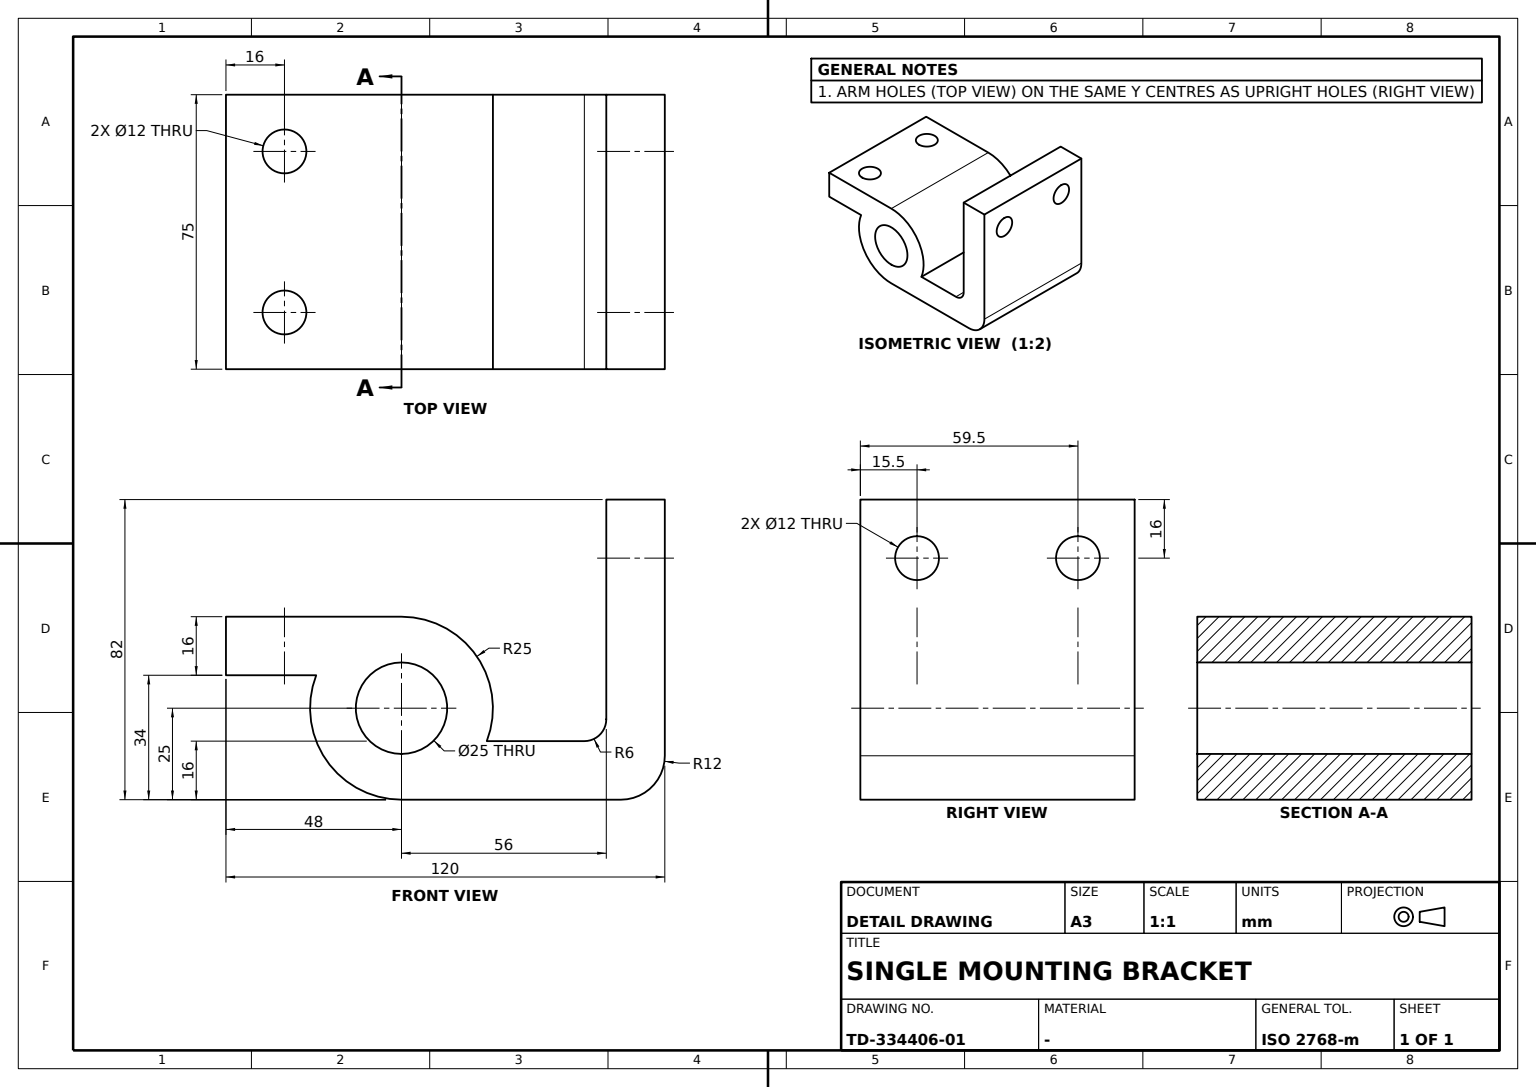
CATIA V5 part; units mm, degrees
sketch "Sketch1" plane through (0, 0, 0) normal (1, 0, 0) x (0, 1, 0)
  arc A0 (-23.3238, 9) -> (0, -25) centre (0, 0) ccw
  circle A1 centre (0, 0) radius 12.5
  line L0 (0, 25) -> (-48, 25)
  line L1 (-48, 25) -> (-48, 9)
  line L2 (-48, 9) -> (-23.3238, 9)
  point P0 (23.3238, -9)
  line L3 (23.3238, -9) -> (56, -9)
  line L4 (56, -9) -> (56, 57)
  line L5 (56, 57) -> (72, 57)
  line L6 (72, 57) -> (72, -25)
  line L7 (72, -25) -> (0, -25)
  arc A2 (23.3238, -9) -> (0, 25) centre (0, 0) ccw
  dimension "radius A0" = 25
  dimension "radius A1" = 12.5
  dimension "length L5" = 16
  dimension "distance L3 L7" = 16
  dimension "length L1" = 16
  dimension "distance L1 L6" = 120
  dimension "distance y axis L4" = 56
  dimension "length L6" = 82
  constraint horizontal L0 x-axis
  constraint horizontal L2 x-axis
  constraint horizontal L3 x-axis
  constraint horizontal L5 x-axis
  constraint horizontal L7 x-axis
  constraint vertical L1 y-axis
  constraint vertical L4 y-axis
  constraint vertical L6 y-axis
  constraint tangency L7 A0
  constraint tangency L0 A0
  constraint coincidence P0 A0
  constraint coincidence A0 A2
extrude "Pad1" add sketch "Sketch1" along normal mid plane 75
fillet "Fillet1" radius 6 1 edges at (0, 56, -9)
fillet "Fillet2" radius 12 1 edges at (0, 72, -25)
sketch "Sketch2" plane through (0, 0, 25) normal (0, 0, 1) x (0, 1, 0)
  circle A0 centre (-32, 22) radius 6
  point P0 (-32, 22)
  line L0 (-48, 37.5) -> (-48, -37.5) construction
  circle A1 centre (-32, -22) radius 6
  dimension "radius A0" = 6
  dimension "distance P0 x axis" = 22
  dimension "distance P0 L0" = 16
  constraint symmetry A0 A1 x-axis
extrude "Pocket1" cut sketch "Sketch2" against normal blind 37.5
sketch "Sketch3" plane through (0, 72, 0) normal (0, 1, 0) x (-1, 0, 0)
  circle A0 centre (-22, 41) radius 6
  point P0 (-22, 41)
  line L0 (37.5, 57) -> (-37.5, 57) construction
  circle A1 centre (22, 41) radius 6
  dimension "radius A0" = 6
  dimension "distance P0 y axis" = 22
  dimension "distance L0 P0" = 16
  constraint symmetry A0 A1 y-axis
extrude "Pocket2" cut sketch "Sketch3" against normal blind 37.5
